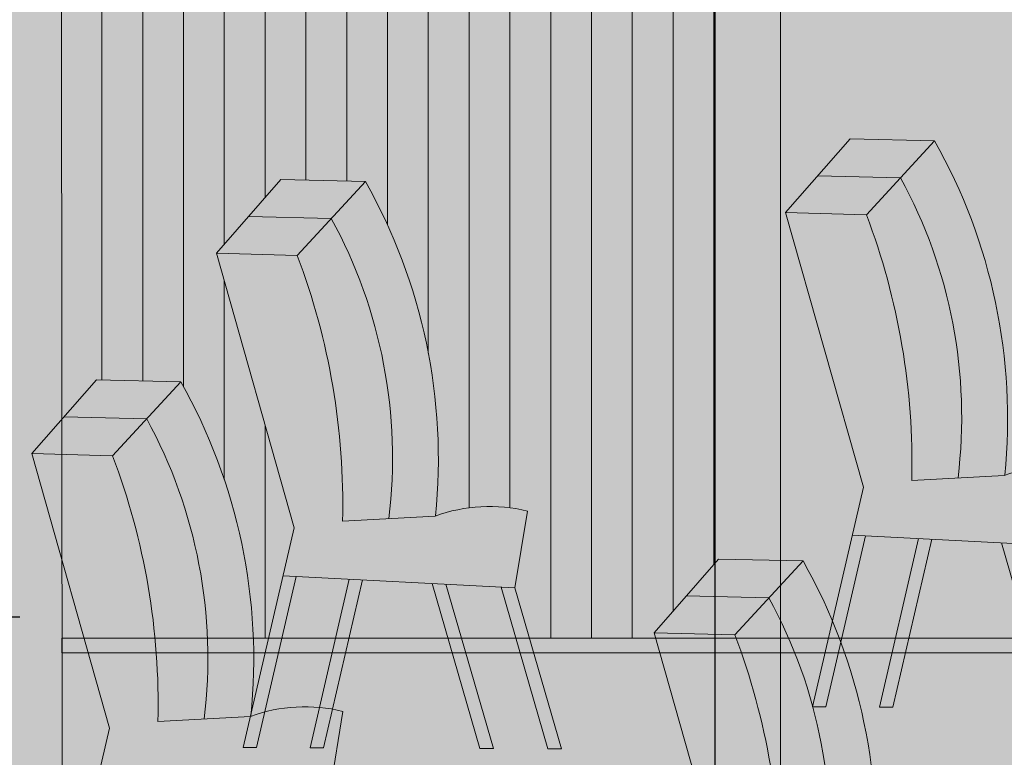
# Model space of a CAD drawing. Units: millimetres. Extents: x 11032 to 26788, y 3406 to 24505.
# Tile 8 of 78: x 15812 to 16566, y 7713 to 8278. Entities that reach past the tile are written whole.
import ezdxf

# ---------------------------------------------------------------- set-up
doc = ezdxf.new("R2010")
doc.units = ezdxf.units.MM
doc.header["$MEASUREMENT"] = 0
for name, color, linetype, lineweight in [('A-ANNO-DIMS', 2, 'Continuous', 18), ('A-FURN', 8, 'Continuous', 13), ('A-FURN-PATT', 8, 'Continuous', 13), ('A-GLAZ', 250, 'Continuous', 20), ('A-WALL-INTR', 8, 'Continuous', 18)]:
    doc.layers.add(name, color=color, linetype=linetype, lineweight=lineweight)
for name, color, linetype, lineweight, true_color in [('A-FNSH-INTR-PATT', 253, 'Continuous', 13, 0xc2b29b), ('A-GLAZ-FRAM-PATT', 250, 'Continuous', 13, 0x262627), ('A-WALL-INTR-PATT', 251, 'Continuous', 13, 0x6c6b6a)]:
    doc.layers.add(name, color=color, linetype=linetype, lineweight=lineweight, true_color=true_color)
doc.styles.get("Standard").update_dxf_attribs({"font": 'arial.ttf'})
doc.dimstyles.get("Standard").update_dxf_attribs({"dimtxt": 150, "dimasz": 100, "dimexe": 10, "dimexo": 5, "dimgap": 5, "dimtad": 0, "dimtih": 1, "dimtoh": 1, "dimdec": 0, "dimzin": 0, "dimdsep": 46, "dimtxsty": 'Standard', "dimcen": 0.09, "dimadec": 0, "dimazin": 0, "dimtfac": 1, "dimtdec": 0, "dimtofl": 0, "dimtmove": 0, "dimatfit": 3, "dimfxl": 1, "dimtolj": 1, "dimtzin": 0, "dimarcsym": 0})

# ---------------------------------------------------------------- blocks, each defined once
blk = doc.blocks.new('DINING-CHAIR-ELEV')
blk.add_line((228.68, 123.43), (51.04, 132.61))
for points in [[(0, 379.55), (49.45, 435.94), (114.12, 434.53)], [(61.18, 132.09), (30.79, 1.16), (20.53, 1.21), (59.55, 169.26), (0, 379.55), (61.9, 377.89)], [(111.9, 129.47), (82.06, 0.91), (71.8, 0.96), (101.76, 129.99)], [(165.28, 126.71), (201.76, 0.31), (212.19, 0.26), (175.85, 126.16)]]:
    blk.add_lwpolyline(points)
for points in [[(218.11, 123.98), (253.88, 0.05), (264.3, 0), (228.68, 123.43), (238.32, 182.18, 0.148451), (167.47, 178.33), (96.61, 174.48, 0.097012), (61.9, 377.89), (114.12, 434.53, -0.154833), (167.82, 178.46)], [(132.04, 176.4, 0.156877), (88.01, 406.21), (24.72, 407.74)]]:
    blk.add_lwpolyline(points, format="xyb")
blk = doc.blocks.new('DINING-TABLE-ELEV')
blk.add_lwpolyline([(0, 0), (986.08, 0), (986.08, 11.1), (0, 11.1)], close=True)
blk = doc.blocks.new('*D16')
at = {"layer": 'A-ANNO-DIMS', "color": 0, "lineweight": -2, "transparency": 16777216}
for p, q in [((15741.74, 7821.05), (15812.13, 7821.05)), ((15802.13, 7721.05), (15802.13, 7685.69)), ((15802.13, 7485.11), (15802.13, 7520.47)), ((15741.74, 7385.11), (15812.13, 7385.11))]:
    blk.add_line(p, q, dxfattribs=at)
at = {"layer": 'A-ANNO-DIMS', "color": 0, "transparency": 16777216}
for points in [[(15785.47, 7721.05), (15818.8, 7721.05), (15802.13, 7821.05)], [(15785.47, 7485.11), (15818.8, 7485.11), (15802.13, 7385.11)]]:
    blk.add_solid(points, dxfattribs=at)
at = {"layer": 'Defpoints', "color": 0, "transparency": 16777216}
for p in [(15736.74, 7821.05), (15802.13, 7821.05), (15736.74, 7385.11)]:
    blk.add_point(p, dxfattribs=at)
at = {"layer": 'A-ANNO-DIMS', "color": 0, "transparency": 16777216, "insert": (15802.13, 7603.08), "char_height": 150, "attachment_point": 5}
blk.add_mtext('\\A1;CHAIR 436 TYP.', dxfattribs=at)
blk = doc.blocks.new('*D36')
at = {"layer": 'A-ANNO-DIMS', "color": 0, "lineweight": -2, "transparency": 16777216}
for p, q in [((12301.26, 17115.89), (12301.26, 24416.86)), ((25397.4, 4466.4), (25397.4, 24416.86)), ((12401.26, 24406.86), (18569.2, 24406.86)), ((25297.4, 24406.86), (19129.47, 24406.86))]:
    blk.add_line(p, q, dxfattribs=at)
at = {"layer": 'A-ANNO-DIMS', "color": 0, "transparency": 16777216}
for points in [[(12401.26, 24423.52), (12401.26, 24390.19), (12301.26, 24406.86)], [(25297.4, 24423.52), (25297.4, 24390.19), (25397.4, 24406.86)]]:
    blk.add_solid(points, dxfattribs=at)
at = {"layer": 'Defpoints', "color": 0, "transparency": 16777216}
for p in [(25397.4, 24406.86), (12301.26, 17110.89), (25397.4, 4461.4)]:
    blk.add_point(p, dxfattribs=at)
at = {"layer": 'A-ANNO-DIMS', "color": 0, "transparency": 16777216, "insert": (18849.33, 24406.86), "char_height": 150, "attachment_point": 5}
blk.add_mtext('\\A1;13096', dxfattribs=at)
blk = doc.blocks.new('*D37')
at = {"layer": 'A-ANNO-DIMS', "color": 0, "lineweight": -2, "transparency": 16777216}
for p, q in [((18087.74, 23450.36), (11334.76, 23450.36)), ((11344.76, 23350.36), (11344.76, 14037.46)), ((11344.76, 4561.4), (11344.76, 13874.29)), ((12927.66, 4461.4), (11334.76, 4461.4))]:
    blk.add_line(p, q, dxfattribs=at)
at = {"layer": 'A-ANNO-DIMS', "color": 0, "transparency": 16777216}
for points in [[(11328.1, 23350.36), (11361.43, 23350.36), (11344.76, 23450.36)], [(11328.1, 4561.4), (11361.43, 4561.4), (11344.76, 4461.4)]]:
    blk.add_solid(points, dxfattribs=at)
at = {"layer": 'Defpoints', "color": 0, "transparency": 16777216}
for p in [(11344.76, 23450.36), (18092.74, 23450.36), (12932.66, 4461.4)]:
    blk.add_point(p, dxfattribs=at)
at = {"layer": 'A-ANNO-DIMS', "color": 0, "transparency": 16777216, "insert": (11344.76, 13955.88), "char_height": 150, "attachment_point": 5}
blk.add_mtext('\\A1;18989', dxfattribs=at)
blk = doc.blocks.new('*D49')
at = {"layer": 'A-ANNO-DIMS', "color": 0, "lineweight": -2, "transparency": 16777216}
for p, q in [((17953.45, 10206.41), (17953.45, 3494.9)), ((14996.4, 6406.4), (14996.4, 3494.9)), ((15096.4, 3504.9), (16244.67, 3504.9)), ((17853.45, 3504.9), (16705.18, 3504.9))]:
    blk.add_line(p, q, dxfattribs=at)
at = {"layer": 'A-ANNO-DIMS', "color": 0, "transparency": 16777216}
for points in [[(15096.4, 3521.57), (15096.4, 3488.23), (14996.4, 3504.9)], [(17853.45, 3521.57), (17853.45, 3488.23), (17953.45, 3504.9)]]:
    blk.add_solid(points, dxfattribs=at)
at = {"layer": 'Defpoints', "color": 0, "transparency": 16777216}
for p in [(17953.45, 10211.41), (14996.4, 6411.4), (17953.45, 3504.9)]:
    blk.add_point(p, dxfattribs=at)
at = {"layer": 'A-ANNO-DIMS', "color": 0, "transparency": 16777216, "insert": (16474.93, 3504.9), "char_height": 150, "attachment_point": 5}
blk.add_mtext('\\A1;2957', dxfattribs=at)
blk = doc.blocks.new('*D57')
at = {"layer": 'A-ANNO-DIMS', "color": 0, "lineweight": -2, "transparency": 16777216}
for p, q in [((14994.7, 7266.4), (14994.7, 24416.86)), ((20894.7, 7266.4), (20894.7, 24416.86)), ((15094.7, 24406.86), (17715.98, 24406.86)), ((20794.7, 24406.86), (18173.42, 24406.86))]:
    blk.add_line(p, q, dxfattribs=at)
at = {"layer": 'A-ANNO-DIMS', "color": 0, "transparency": 16777216}
for points in [[(15094.7, 24423.52), (15094.7, 24390.19), (14994.7, 24406.86)], [(20794.7, 24423.52), (20794.7, 24390.19), (20894.7, 24406.86)]]:
    blk.add_solid(points, dxfattribs=at)
at = {"layer": 'Defpoints', "color": 0, "transparency": 16777216}
for p in [(20894.7, 24406.86), (14994.7, 7261.4), (20894.7, 7261.4)]:
    blk.add_point(p, dxfattribs=at)
at = {"layer": 'A-ANNO-DIMS', "color": 0, "transparency": 16777216, "insert": (17944.7, 24406.86), "char_height": 150, "attachment_point": 5}
blk.add_mtext('\\A1;5900', dxfattribs=at)
blk = doc.blocks.new('*D60')
at = {"layer": 'A-ANNO-DIMS', "color": 0, "lineweight": -2, "transparency": 16777216}
for p, q in [((14994.7, 7266.4), (14994.7, 24416.86)), ((16344.7, 7266.4), (16344.7, 24416.86)), ((15094.7, 24406.86), (15448.04, 24406.86)), ((16244.7, 24406.86), (15891.36, 24406.86))]:
    blk.add_line(p, q, dxfattribs=at)
at = {"layer": 'A-ANNO-DIMS', "color": 0, "transparency": 16777216}
for points in [[(15094.7, 24423.52), (15094.7, 24390.19), (14994.7, 24406.86)], [(16244.7, 24423.52), (16244.7, 24390.19), (16344.7, 24406.86)]]:
    blk.add_solid(points, dxfattribs=at)
at = {"layer": 'Defpoints', "color": 0, "transparency": 16777216}
for p in [(16344.7, 24406.86), (14994.7, 7261.4), (16344.7, 7261.4)]:
    blk.add_point(p, dxfattribs=at)
at = {"layer": 'A-ANNO-DIMS', "color": 0, "transparency": 16777216, "insert": (15669.7, 24406.86), "char_height": 150, "attachment_point": 5}
blk.add_mtext('\\A1;1350', dxfattribs=at)
blk = doc.blocks.new('*D69')
at = {"layer": 'A-ANNO-DIMS', "color": 0, "lineweight": -2, "transparency": 16777216}
for p, q in [((13956.97, 9937.95), (14056.97, 9937.95)), ((14056.97, 9937.95), (15432.5, 8990.95)), ((17944.61, 7261.4), (17944.79, 7261.4)), ((17944.7, 7261.31), (17944.7, 7261.49))]:
    blk.add_line(p, q, dxfattribs=at)
at = {"layer": 'A-ANNO-DIMS', "color": 0, "transparency": 16777216}
blk.add_solid([(15441.95, 9004.68), (15423.05, 8977.22), (15514.87, 8934.24)], dxfattribs=at)
at = {"layer": 'Defpoints', "color": 0, "transparency": 16777216}
for p in [(15514.87, 8934.24), (17944.7, 7261.4)]:
    blk.add_point(p, dxfattribs=at)
at = {"layer": 'A-ANNO-DIMS', "color": 0, "transparency": 16777216, "insert": (13494.04, 9937.95), "char_height": 150, "attachment_point": 5}
blk.add_mtext('\\A1;2X R2950', dxfattribs=at)

msp = doc.modelspace()

# ---------------------------------------------------------------- hatches: boundary and pattern name
at = {"layer": 'A-FNSH-INTR-PATT'}
h = msp.add_hatch(dxfattribs=at)
h.set_pattern_fill('ANSI31', color=256, scale=250, angle=45, style=0)
h.paths.add_polyline_path([(16344.704, 9680.076, 0.0565356), (15843.607, 9260.247), (15844.323, 7974.176), (15846.037, 7974.134), (15870.762, 8002.329), (15935.434, 8000.923, -0.1195917), (15991.005, 7804.617), (16002.667, 7804.617), (16022.264, 7889.032), (15962.718, 8099.323), (16012.167, 8155.712), (16076.839, 8154.307, -0.1548334), (16130.535, 7898.229, -0.1476694), (16201.035, 7901.954), (16191.395, 7843.208), (16202.533, 7804.617), (16299.12, 7804.617), (16297.929, 7808.825), (16344.704, 7862.164)])
at = {"layer": 'A-FURN-PATT'}
h = msp.add_hatch(color=256, dxfattribs=at)
h.set_gradient(color1=(82, 15, 16), color2=(153, 0, 38), name='CURVED')
h.paths.add_polyline_path([(16952.125, 8119), (16926.017, 8147.32, 0.1568775), (16881.989, 7917.509), (16917.415, 7915.583, -0.0970121)], flags=0)
h.paths.add_polyline_path([(16899.908, 8175.64), (16964.58, 8177.046), (17014.03, 8120.657), (16954.484, 7910.365), (16972.017, 7834.84), (16977.75, 7834.965), (17027.199, 7778.576), (16967.653, 7568.284), (17006.665, 7400.238), (16996.411, 7400.187), (16966.016, 7531.114), (16925.439, 7529.018), (16955.395, 7399.983), (16945.141, 7399.932), (16915.295, 7528.494), (16861.916, 7525.736), (16825.435, 7399.337), (16815.012, 7399.285), (16851.35, 7525.19), (16809.087, 7523.007), (16773.319, 7399.078), (16762.896, 7399.026), (16798.521, 7522.461), (16788.882, 7581.207, -0.1476694), (16859.382, 7577.482, -0.1528132), (16911.41, 7830.579), (16902.125, 7870.575), (16848.746, 7867.817), (16830.506, 7804.617), (16830.506, 7793.515), (16827.302, 7793.515), (16812.265, 7741.418), (16801.842, 7741.366), (16816.893, 7793.515), (16775.261, 7793.515), (16760.15, 7741.159), (16749.727, 7741.107), (16764.853, 7793.515), (16650.704, 7793.515), (16662.994, 7750.932), (16652.571, 7750.983), (16640.296, 7793.515), (16598.663, 7793.515), (16610.879, 7751.191), (16600.455, 7751.242), (16588.255, 7793.515), (16490.425, 7793.515), (16480.749, 7751.837), (16470.495, 7751.888), (16480.159, 7793.515), (16443.833, 7793.515, -0.1094051), (16465.746, 7607.731, -0.1476694), (16536.246, 7611.456), (16526.606, 7552.71), (16562.232, 7429.275), (16551.809, 7429.327), (16516.041, 7553.255), (16473.778, 7555.439), (16510.116, 7429.534), (16499.693, 7429.586), (16463.212, 7555.985), (16409.833, 7558.743), (16379.987, 7430.181), (16369.733, 7430.232), (16394.704, 7537.793), (16394.704, 7559.524), (16359.112, 7561.363), (16328.717, 7430.435), (16318.463, 7430.486), (16344.704, 7543.521), (16344.704, 7643.635), (16302.264, 7793.515), (16205.738, 7793.515), (16227.021, 7719.773), (16216.598, 7719.825), (16195.329, 7793.515), (16153.697, 7793.515), (16174.905, 7720.032), (16164.482, 7720.084), (16143.289, 7793.515), (15844.423, 7793.515), (15844.423, 7804.617), (16140.084, 7804.617), (16128.001, 7846.483), (16191.395, 7843.208), (16201.035, 7901.954, 0.1484508), (16130.184, 7898.102), (16059.333, 7894.25, 0.0970121), (16024.622, 8097.666), (16076.839, 8154.307, -0.1548334), (16130.535, 7898.229, -0.1476694), (16201.035, 7901.954), (16191.395, 7843.208), (16202.533, 7804.617), (16299.12, 7804.617), (16297.929, 7808.825), (16347.378, 7865.214), (16412.05, 7863.808, -0.0295496), (16434.494, 7817.915), (16458.237, 7920.19), (16398.691, 8130.481), (16448.141, 8186.871), (16512.813, 8185.465, -0.1548334), (16566.508, 7929.387, -0.1476694), (16637.008, 7933.112), (16627.369, 7874.366), (16647.499, 7804.617), (16742.939, 7804.617), (16741.107, 8264.696), (17994.704, 8264.696), (17994.704, 7796.661), (18112.02, 7796.661), (18134.447, 7874.366), (18124.807, 7933.112, -0.1476694), (18195.307, 7929.387, -0.1548334), (18249.003, 8185.465), (18313.675, 8186.871), (18363.124, 8130.481), (18303.578, 7920.19), (18311.087, 7887.847, -0.0273017), (18332.016, 7930.161), (18396.688, 7931.567), (18446.137, 7875.177), (18423.905, 7796.661), (18470.25, 7796.661), (18470.25, 7785.559), (18420.761, 7785.559), (18386.591, 7664.886), (18425.604, 7496.839), (18415.35, 7496.788), (18384.955, 7627.716), (18344.377, 7625.62), (18374.333, 7496.584), (18364.079, 7496.533), (18334.233, 7625.095), (18280.854, 7622.338), (18244.373, 7495.938), (18233.95, 7495.887), (18270.288, 7621.792), (18228.026, 7619.608), (18192.257, 7495.679), (18181.834, 7495.628), (18217.46, 7619.062), (18207.82, 7677.808, -0.1476694), (18278.32, 7674.083, -0.0514181), (18278.516, 7762.821), (18273.237, 7785.559), (18171.265, 7785.559), (18161.36, 7751.242), (18150.937, 7751.191), (18160.856, 7785.559), (18119.224, 7785.559), (18109.244, 7750.983), (18098.821, 7750.932), (18108.815, 7785.559), (17852.794, 7785.559), (17866.18, 7739.181), (17855.756, 7739.233), (17842.386, 7785.559), (17800.753, 7785.559), (17814.064, 7739.44), (17803.641, 7739.492), (17790.345, 7785.559), (17694.491, 7785.559), (17685.986, 7748.922, -0.0882745), (17728.687, 7746.171), (17719.047, 7687.425), (17754.673, 7563.99), (17744.25, 7564.042), (17708.482, 7687.971), (17666.219, 7690.154), (17702.557, 7564.249), (17692.134, 7564.301), (17655.653, 7690.7), (17602.274, 7693.458), (17572.428, 7564.896), (17562.174, 7564.947), (17592.13, 7693.982), (17551.553, 7696.078), (17521.158, 7565.151), (17510.903, 7565.202), (17549.916, 7733.248), (17535.103, 7785.559), (17484.167, 7785.559), (17484.167, 7796.661), (17531.96, 7796.661), (17490.37, 7943.54), (17539.819, 7999.929), (17604.491, 7998.523, -0.0802486), (17652.289, 7869.096), (17661.422, 7908.439), (17601.876, 8118.731), (17651.326, 8175.12), (17715.998, 8173.714, -0.1548334), (17769.694, 7917.637, -0.1476694), (17840.194, 7921.361), (17830.554, 7862.615), (17849.59, 7796.661), (17894.704, 7796.661), (17894.704, 8239.696), (16741.207, 8239.696), (16742.939, 7804.617), (16768.057, 7804.617), (16785.352, 7864.542), (16775.713, 7923.288, -0.1476694), (16846.212, 7919.563, -0.1548334)], flags=17)
h.paths.add_polyline_path([(16899.908, 8175.64), (16964.58, 8177.046), (17014.03, 8120.657), (16954.484, 7910.365), (16993.496, 7742.318), (16983.242, 7742.267), (16952.847, 7873.195), (16912.27, 7871.099), (16942.225, 7742.064), (16931.971, 7742.013), (16902.125, 7870.575), (16848.746, 7867.817), (16812.265, 7741.418), (16801.842, 7741.366), (16838.181, 7867.271), (16795.918, 7865.087), (16760.15, 7741.159), (16749.727, 7741.107), (16785.352, 7864.542), (16775.713, 7923.288, -0.1476694), (16846.212, 7919.563, -0.1548334)], flags=0)
h.paths.add_polyline_path([(16899.908, 8175.64), (16964.58, 8177.046), (17014.03, 8120.657), (16954.484, 7910.365), (16972.017, 7834.84), (16977.75, 7834.965), (17027.199, 7778.576), (16967.653, 7568.284), (17006.665, 7400.238), (16996.411, 7400.187), (16966.016, 7531.114), (16925.439, 7529.018), (16955.395, 7399.983), (16945.141, 7399.932), (16915.295, 7528.494), (16861.916, 7525.736), (16825.435, 7399.337), (16815.012, 7399.285), (16851.35, 7525.19), (16809.087, 7523.007), (16773.319, 7399.078), (16762.896, 7399.026), (16798.521, 7522.461), (16788.882, 7581.207, -0.1476694), (16859.382, 7577.482, -0.1528132), (16911.41, 7830.579), (16902.125, 7870.575), (16848.746, 7867.817), (16830.506, 7804.617), (16830.506, 7793.515), (16827.302, 7793.515), (16812.265, 7741.418), (16801.842, 7741.366), (16816.893, 7793.515), (16775.261, 7793.515), (16760.15, 7741.159), (16749.727, 7741.107), (16764.853, 7793.515), (16650.704, 7793.515), (16662.994, 7750.932), (16652.571, 7750.983), (16640.296, 7793.515), (16598.663, 7793.515), (16610.879, 7751.191), (16600.455, 7751.242), (16588.255, 7793.515), (16490.425, 7793.515), (16480.749, 7751.837), (16470.495, 7751.888), (16480.159, 7793.515), (16443.833, 7793.515, -0.1094051), (16465.746, 7607.731, -0.1476694), (16536.246, 7611.456), (16526.606, 7552.71), (16562.232, 7429.275), (16551.809, 7429.327), (16516.041, 7553.255), (16473.778, 7555.439), (16510.116, 7429.534), (16499.693, 7429.586), (16463.212, 7555.985), (16409.833, 7558.743), (16379.987, 7430.181), (16369.733, 7430.232), (16394.704, 7537.793), (16394.704, 7559.524), (16359.112, 7561.363), (16328.717, 7430.435), (16318.463, 7430.486), (16344.704, 7543.521), (16344.704, 7643.635), (16302.264, 7793.515), (16205.738, 7793.515), (16227.021, 7719.773), (16216.598, 7719.825), (16195.329, 7793.515), (16153.697, 7793.515), (16174.905, 7720.032), (16164.482, 7720.084), (16143.289, 7793.515), (15844.423, 7793.515), (15844.423, 7804.617), (16140.084, 7804.617), (16128.001, 7846.483), (16191.395, 7843.208), (16201.035, 7901.954, 0.1484508), (16130.184, 7898.102), (16059.333, 7894.25, 0.0970121), (16024.622, 8097.666), (16076.839, 8154.307, -0.1548334), (16130.535, 7898.229, -0.1476694), (16201.035, 7901.954), (16191.395, 7843.208), (16202.533, 7804.617), (16299.12, 7804.617), (16297.929, 7808.825), (16347.378, 7865.214), (16412.05, 7863.808, -0.0295496), (16434.494, 7817.915), (16458.237, 7920.19), (16398.691, 8130.481), (16448.141, 8186.871), (16512.813, 8185.465, -0.1548334), (16566.508, 7929.387, -0.1476694), (16637.008, 7933.112), (16627.369, 7874.366), (16647.499, 7804.617), (16742.939, 7804.617), (16741.207, 8239.696), (16741.107, 8264.696), (17994.704, 8264.696), (17994.704, 7796.661), (18112.02, 7796.661), (18134.447, 7874.366), (18124.807, 7933.112, -0.1476694), (18195.307, 7929.387, -0.1548334), (18249.003, 8185.465), (18313.675, 8186.871), (18363.124, 8130.481), (18303.578, 7920.19), (18311.087, 7887.847, -0.0273017), (18332.016, 7930.161), (18396.688, 7931.567), (18446.137, 7875.177), (18423.905, 7796.661), (18470.25, 7796.661), (18470.25, 7785.559), (18420.761, 7785.559), (18386.591, 7664.886), (18425.604, 7496.839), (18415.35, 7496.788), (18384.955, 7627.716), (18344.377, 7625.62), (18374.333, 7496.584), (18364.079, 7496.533), (18334.233, 7625.095), (18280.854, 7622.338), (18244.373, 7495.938), (18233.95, 7495.887), (18270.288, 7621.792), (18228.026, 7619.608), (18192.257, 7495.679), (18181.834, 7495.628), (18217.46, 7619.062), (18207.82, 7677.808, -0.1476694), (18278.32, 7674.083, -0.0514181), (18278.516, 7762.821), (18273.237, 7785.559), (18171.265, 7785.559), (18161.36, 7751.242), (18150.937, 7751.191), (18160.856, 7785.559), (18119.224, 7785.559), (18109.244, 7750.983), (18098.821, 7750.932), (18108.815, 7785.559), (17852.794, 7785.559), (17866.18, 7739.181), (17855.756, 7739.233), (17842.386, 7785.559), (17800.753, 7785.559), (17814.064, 7739.44), (17803.641, 7739.492), (17790.345, 7785.559), (17694.491, 7785.559), (17685.986, 7748.922, -0.0882745), (17728.687, 7746.171), (17719.047, 7687.425), (17754.673, 7563.99), (17744.25, 7564.042), (17708.482, 7687.971), (17666.219, 7690.154), (17702.557, 7564.249), (17692.134, 7564.301), (17655.653, 7690.7), (17602.274, 7693.458), (17572.428, 7564.896), (17562.174, 7564.947), (17592.13, 7693.982), (17551.553, 7696.078), (17521.158, 7565.151), (17510.903, 7565.202), (17549.916, 7733.248), (17535.103, 7785.559), (17484.167, 7785.559), (17484.167, 7796.661), (17531.96, 7796.661), (17490.37, 7943.54), (17539.819, 7999.929), (17604.491, 7998.523, -0.0802486), (17652.289, 7869.096), (17661.422, 7908.439), (17601.876, 8118.731), (17651.326, 8175.12), (17715.998, 8173.714, -0.1548334), (17769.694, 7917.637, -0.1476694), (17840.194, 7921.361), (17830.554, 7862.615), (17849.59, 7796.661), (17894.704, 7796.661), (17894.704, 8239.696), (16741.207, 8239.696), (16742.939, 7804.617), (16768.057, 7804.617), (16785.352, 7864.542), (16775.713, 7923.288, -0.1476694), (16846.212, 7919.563, -0.1548334)], flags=17)
h = msp.add_hatch(color=256, dxfattribs=at)
h.set_gradient(color1=(153, 27, 30), color2=(153, 38, 0), name='SPHERICAL')
h.paths.add_polyline_path([(15534.344, 7763), (15472.44, 7764.657), (15531.986, 7554.365), (15523.479, 7517.719), (15640.736, 7511.661), (15653.713, 7567.556, 0.0295203), (15639.906, 7563.436), (15569.055, 7559.583, 0.0970121)], flags=16)
h.paths.add_polyline_path([(15560.453, 7791.32), (15534.344, 7763, -0.0970121), (15569.055, 7559.583), (15604.48, 7561.509, 0.1568775)], flags=16)
h.paths.add_polyline_path([(15586.562, 7819.64), (15560.453, 7791.32, -0.1568775), (15604.48, 7561.509), (15640.246, 7563.454, 0.154898)], flags=17)
h.paths.add_polyline_path([(15560.453, 7791.32), (15497.165, 7792.851), (15472.44, 7764.657), (15534.344, 7763)], flags=16)
h.paths.add_polyline_path([(15586.562, 7819.64), (15521.889, 7821.046), (15497.165, 7792.851), (15560.453, 7791.32)], flags=17)
h.paths.add_polyline_path([(15790.874, 7662.689, 0.021469), (15780.879, 7659.53), (15710.028, 7655.677, 0.0970121), (15675.317, 7859.094), (15665.772, 7859.35), (15665.799, 7675.745), (15672.959, 7650.459), (15665.807, 7619.654), (15665.808, 7613.744), (15790.755, 7607.288)], flags=17)
h.paths.add_polyline_path([(15665.772, 7859.35), (15613.413, 7860.751), (15665.799, 7675.745)], flags=16)
h.paths.add_polyline_path([(15701.426, 7887.414), (15665.767, 7888.277), (15665.772, 7859.35), (15675.317, 7859.094)], flags=16)
h.paths.add_polyline_path([(15727.534, 7915.735), (15665.763, 7917.077), (15665.767, 7888.277), (15701.426, 7887.414)], flags=17)
h.paths.add_polyline_path([(15665.763, 7917.077), (15662.862, 7917.14), (15638.137, 7888.946), (15665.767, 7888.277)], flags=17)
h.paths.add_polyline_path([(15665.767, 7888.277), (15638.137, 7888.946), (15613.413, 7860.751), (15665.772, 7859.35)], flags=16)
h.paths.add_polyline_path([(15701.426, 7887.414), (15675.317, 7859.094, -0.0970121), (15710.028, 7655.677), (15745.453, 7657.604, 0.1568775)], flags=16)
h.paths.add_polyline_path([(15844.495, 7664.925), (15844.384, 7864.461), (15821.312, 7945.94), (15870.762, 8002.329), (15935.434, 8000.923, -0.1195917), (15991.005, 7804.617), (16002.667, 7804.617), (16022.264, 7889.032), (15962.718, 8099.323), (16024.622, 8097.666), (16076.839, 8154.307, -0.1548334), (16130.535, 7898.229, -0.1476694), (16201.035, 7901.954), (16191.395, 7843.208), (16202.533, 7804.617), (16299.12, 7804.617), (16297.929, 7808.825), (16347.378, 7865.214), (16412.05, 7863.808, -0.0295496), (16434.494, 7817.915), (16458.237, 7920.19), (16398.691, 8130.481), (16460.595, 8128.825), (16512.813, 8185.465, -0.1548334), (16566.508, 7929.387, -0.1476694), (16637.008, 7933.112), (16627.369, 7874.366), (16647.499, 7804.617), (16830.506, 7804.617), (16830.506, 7793.515), (16650.704, 7793.515), (16662.994, 7750.932), (16652.571, 7750.983), (16640.296, 7793.515), (16490.425, 7793.515), (16480.749, 7751.837), (16470.495, 7751.888), (16480.159, 7793.515), (16443.833, 7793.515, -0.1094051), (16465.746, 7607.731, -0.1476694), (16536.246, 7611.456), (16526.606, 7552.71), (16562.232, 7429.275), (16551.809, 7429.327), (16516.041, 7553.255), (16473.778, 7555.439), (16510.116, 7429.534), (16499.693, 7429.586), (16463.212, 7555.985), (16409.833, 7558.743), (16379.987, 7430.181), (16369.733, 7430.232), (16394.704, 7537.793), (16394.704, 7559.524), (16359.112, 7561.363), (16328.717, 7430.435), (16318.463, 7430.486), (16344.704, 7543.521), (16344.704, 7643.635), (16302.264, 7793.515), (16205.738, 7793.515), (16227.021, 7719.773), (16216.598, 7719.825), (16195.329, 7793.515), (16153.697, 7793.515), (16174.905, 7720.032), (16164.482, 7720.084), (16143.289, 7793.515), (16061.685, 7793.515), (16051.641, 7750.248, -0.0167144), (16059.629, 7748.571), (16049.99, 7689.825), (16085.615, 7566.39), (16075.192, 7566.442), (16039.424, 7690.371), (15997.161, 7692.554), (16033.5, 7566.649), (16023.077, 7566.701), (15986.595, 7693.1), (15933.216, 7695.858), (15903.371, 7567.296), (15893.116, 7567.347), (15923.072, 7696.382), (15882.495, 7698.478), (15852.409, 7568.882), (15877.716, 7481.201), (15867.293, 7481.253), (15842.372, 7567.599), (15841.846, 7567.602), (15842.08, 7568.609), (15831.524, 7605.182), (15790.755, 7607.288), (15790.744, 7602.228), (15825.6, 7481.46), (15815.177, 7481.512), (15778.696, 7607.911), (15725.317, 7610.669), (15701.389, 7507.6), (15736.743, 7385.107), (15726.32, 7385.159), (15696.749, 7487.614), (15695.471, 7482.107), (15685.217, 7482.158), (15691.06, 7507.327), (15690.552, 7509.088), (15650.881, 7511.137), (15649.743, 7506.234), (15684.627, 7385.366), (15674.204, 7385.418), (15645.103, 7486.248), (15644.2, 7482.362), (15633.946, 7482.413), (15639.413, 7505.961), (15637.723, 7511.817), (15584.344, 7514.575), (15554.498, 7386.013), (15544.244, 7386.064), (15574.2, 7515.099), (15533.623, 7517.195), (15503.228, 7386.268), (15492.974, 7386.319), (15531.986, 7554.365), (15472.44, 7764.657), (15497.165, 7792.851), (15521.889, 7821.046), (15586.562, 7819.64, -0.1548334), (15640.257, 7563.563, -0.0287549), (15653.713, 7567.556), (15665.807, 7619.654), (15665.799, 7675.745), (15613.413, 7860.751), (15638.137, 7888.946), (15662.862, 7917.14), (15665.763, 7917.077), (15727.534, 7915.735, -0.1548334), (15781.23, 7659.657, -0.1322263)])
h = msp.add_hatch(color=256, dxfattribs=at)
h.set_gradient(color1=(153, 27, 30), color2=(153, 38, 0), name='SPHERICAL')
h.paths.add_polyline_path([(16050.731, 8125.986), (15987.442, 8127.518), (15962.718, 8099.323), (16024.622, 8097.666)])
h.paths.add_polyline_path([(16076.839, 8154.307), (16012.167, 8155.712), (15987.442, 8127.518), (16050.731, 8125.986)])
h.paths.add_polyline_path([(16486.704, 8157.145), (16423.416, 8158.676), (16398.691, 8130.481), (16460.595, 8128.825)])
h.paths.add_polyline_path([(16512.813, 8185.465), (16448.141, 8186.871), (16423.416, 8158.676), (16486.704, 8157.145)])
h = msp.add_hatch(color=256, dxfattribs=at)
h.set_gradient(color1=(153, 27, 30), color2=(153, 38, 0), name='SPHERICAL')
h.paths.add_polyline_path([(15710.028, 7655.677), (15745.453, 7657.604, 0.1568775), (15701.426, 7887.414), (15675.317, 7859.094, -0.0970121)], flags=16)
h.paths.add_polyline_path([(15790.755, 7607.288), (15790.874, 7662.689, 0.021469), (15780.879, 7659.53), (15710.028, 7655.677, 0.0970121), (15675.317, 7859.094), (15665.772, 7859.35), (15665.799, 7675.745), (15672.959, 7650.459), (15665.807, 7619.654), (15665.808, 7613.744)], flags=17)
h.paths.add_polyline_path([(15653.713, 7567.556), (15665.807, 7619.654), (15665.799, 7675.745), (15613.413, 7860.751), (15662.862, 7917.14), (15727.534, 7915.735, -0.1548334), (15781.23, 7659.657, -0.1322263), (15844.495, 7664.925), (15844.384, 7864.461), (15821.312, 7945.94), (15883.216, 7944.283), (15935.434, 8000.923, -0.1195917), (15991.005, 7804.617), (16002.667, 7804.617), (16022.264, 7889.032), (15962.718, 8099.323), (16024.622, 8097.666), (16076.839, 8154.307, -0.1548334), (16130.535, 7898.229, -0.1476694), (16201.035, 7901.954), (16191.395, 7843.208), (16202.533, 7804.617), (16830.506, 7804.617), (16830.506, 7793.515), (16205.738, 7793.515), (16227.021, 7719.773), (16216.598, 7719.825), (16195.329, 7793.515), (16153.697, 7793.515), (16174.905, 7720.032), (16164.482, 7720.084), (16143.289, 7793.515), (16061.685, 7793.515), (16051.641, 7750.248, -0.0167144), (16059.629, 7748.571), (16049.99, 7689.825), (16085.615, 7566.39), (16075.192, 7566.442), (16039.424, 7690.371), (15997.161, 7692.554), (16033.5, 7566.649), (16023.077, 7566.701), (15986.595, 7693.1), (15933.216, 7695.858), (15903.371, 7567.296), (15893.116, 7567.347), (15923.072, 7696.382), (15882.495, 7698.478), (15852.409, 7568.882), (15877.716, 7481.201), (15867.293, 7481.253), (15842.372, 7567.599), (15841.846, 7567.602), (15842.08, 7568.609), (15831.524, 7605.182), (15790.755, 7607.288), (15790.744, 7602.228), (15825.6, 7481.46), (15815.177, 7481.512), (15778.696, 7607.911), (15725.317, 7610.669), (15701.389, 7507.6), (15736.743, 7385.107), (15726.32, 7385.159), (15696.749, 7487.614), (15695.471, 7482.107), (15685.217, 7482.158), (15705.262, 7568.502, 0.0841685), (15664.448, 7569.579), (15644.2, 7482.362), (15633.946, 7482.413), (15653.713, 7567.556, 0.0295203), (15639.906, 7563.436), (15569.055, 7559.583, 0.0970121), (15534.344, 7763), (15472.44, 7764.657), (15521.889, 7821.046), (15586.562, 7819.64, -0.1548334), (15640.257, 7563.563, -0.0287549)])
at = {"layer": 'A-GLAZ-FRAM-PATT'}
h = msp.add_hatch(color=256, dxfattribs=at)
h.paths.add_polyline_path([(17944.704, 7311.399), (16344.704, 7311.399), (16344.704, 7261.399), (17944.704, 7261.399)], flags=17)
h.paths.add_polyline_path([(16344.704, 7311.399), (15045.135, 7311.399, -0.9829047), (20844.273, 7311.399), (19544.704, 7311.399), (19544.704, 7261.399), (20894.704, 7261.399, 0.5148441), (16985.951, 10051.255, 0.3202679), (14994.704, 7261.399), (16344.704, 7261.399)])
h.paths.add_polyline_path([(18744.704, 7311.399), (17944.704, 7311.399), (17944.704, 7261.399), (18744.704, 7261.399)], flags=17)
h.paths.add_polyline_path([(19544.704, 7311.399), (18744.704, 7311.399), (18744.704, 7261.399), (19544.704, 7261.399)], flags=17)
h.paths.add_polyline_path([(18694.704, 7361.399), (17994.704, 7361.399), (17994.704, 7311.399), (18694.704, 7311.399)], flags=17)
h.paths.add_polyline_path([(18744.704, 7361.399), (18694.704, 7361.399), (18694.704, 7311.399), (18744.704, 7311.399)], flags=17)
h.paths.add_polyline_path([(17194.704, 7361.399), (17144.704, 7361.399), (17144.704, 7311.399), (17194.704, 7311.399)], flags=17)
h.paths.add_polyline_path([(17431.432, 7361.399), (17194.704, 7361.399), (17194.704, 7311.399), (17431.699, 7311.399)], flags=17)
h.paths.add_polyline_path([(17894.704, 7361.399), (17431.432, 7361.399), (17431.699, 7311.399), (17894.704, 7311.399)], flags=17)
h.paths.add_polyline_path([(17944.704, 7361.399), (17894.704, 7361.399), (17894.704, 7311.399), (17944.704, 7311.399)], flags=17)
h.paths.add_polyline_path([(17994.704, 7361.399), (17944.704, 7361.399), (17944.704, 7311.399), (17994.704, 7311.399)], flags=17)
h = msp.add_hatch(color=256, dxfattribs=at)
h.paths.add_polyline_path([(16394.704, 9712.419, 0.0051337), (16344.704, 9680.076), (16344.704, 7862.164), (16347.378, 7865.214), (16394.704, 7864.185)])
h.paths.add_polyline_path([(17144.704, 10048.871, 0.0235225), (16886.403, 9961.399), (17094.704, 9961.399), (17094.704, 8264.696), (17144.704, 8264.696)])
h.paths.add_polyline_path([(18794.704, 9961.399), (19003.004, 9961.399, 0.0235225), (18744.704, 10048.871), (18744.704, 8264.696), (18794.704, 8264.696)])
h.paths.add_polyline_path([(19544.704, 9680.076, 0.0051337), (19494.704, 9712.419), (19494.704, 7793.43), (19544.704, 7793.43)])
h = msp.add_hatch(color=256, dxfattribs=at)
h.paths.add_polyline_path([(16734.609, 9896.863, 0.0333754), (16394.704, 9712.419), (16394.704, 7804.617), (16431.407, 7804.617), (16458.237, 7920.19), (16398.691, 8130.481), (16448.141, 8186.871), (16512.813, 8185.465, -0.1548334), (16566.508, 7929.387, -0.1476694), (16637.008, 7933.112), (16627.369, 7874.366), (16647.499, 7804.617), (16742.939, 7804.617)])
h.paths.add_polyline_path([(17094.704, 9961.399), (16886.403, 9961.399, 0.0142221), (16734.609, 9896.863), (16741.107, 8264.696), (17094.704, 8264.696)])
h.paths.add_polyline_path([(17417.202, 10027.292), (17194.704, 10011.399), (17194.704, 8264.696), (17426.61, 8264.696)])
h.paths.add_polyline_path([(17144.704, 8239.696), (17094.704, 8239.696), (17094.704, 7361.399), (16394.704, 7361.399), (16394.704, 7493.572), (16379.987, 7430.181), (16369.733, 7430.232), (16394.704, 7537.793), (16394.704, 7559.524), (16359.112, 7561.363), (16344.704, 7499.3), (16344.704, 7311.399), (17144.704, 7311.399)])
h.paths.add_polyline_path([(17194.704, 8239.696), (17144.704, 8239.696), (17144.704, 7361.399), (17194.704, 7361.399)])
at = {"layer": 'A-WALL-INTR-PATT'}
for points in [[(16344.704, 9680.076, 0.0565356), (15843.607, 9260.247), (15844.323, 7974.176), (15846.037, 7974.134), (15870.762, 8002.329), (15935.434, 8000.923, -0.1195917), (15991.005, 7804.617), (16002.667, 7804.617), (16022.264, 7889.032), (15962.718, 8099.323), (16012.167, 8155.712), (16076.839, 8154.307, -0.1548334), (16130.535, 7898.229, -0.1476694), (16201.035, 7901.954), (16191.395, 7843.208), (16202.533, 7804.617), (16299.12, 7804.617), (16297.929, 7808.825), (16344.704, 7862.164)], [(15843.607, 9260.247, 0.0062633), (15794.195, 9206.987), (15790.874, 7662.689, -0.1112179), (15844.495, 7664.925), (15844.384, 7864.461), (15821.312, 7945.94), (15844.324, 7972.181)]]:
    msp.add_hatch(color=256, dxfattribs=at).paths.add_polyline_path(points)
h = msp.add_hatch(color=256, dxfattribs=at)
h.paths.add_polyline_path([(15302.659, 8457.059, 0.0281002), (15185.248, 8153.253), (15233.282, 7717.599), (15314.374, 7311.399), (15467.334, 7311.399), (15381.661, 7740.545)])
h.paths.add_polyline_path([(16344.704, 7543.521), (16344.704, 7643.635), (16302.264, 7793.515), (16205.738, 7793.515), (16227.021, 7719.773), (16216.598, 7719.825), (16195.329, 7793.515), (16153.697, 7793.515), (16174.905, 7720.032), (16164.482, 7720.084), (16143.289, 7793.515), (16061.685, 7793.515), (16051.641, 7750.248, -0.0167144), (16059.629, 7748.571), (16049.99, 7689.825), (16085.615, 7566.39), (16075.192, 7566.442), (16039.424, 7690.371), (15997.161, 7692.554), (16033.5, 7566.649), (16023.077, 7566.701), (15986.595, 7693.1), (15933.216, 7695.858), (15903.371, 7567.296), (15893.116, 7567.347), (15923.072, 7696.382), (15882.495, 7698.478), (15852.409, 7568.882), (15877.716, 7481.201), (15867.293, 7481.253), (15844.553, 7560.041), (15844.691, 7311.399), (16344.704, 7311.399), (16344.704, 7499.3), (16328.717, 7430.435), (16318.463, 7430.486)])
h.paths.add_polyline_path([(16742.983, 7793.515), (16650.704, 7793.515), (16662.994, 7750.932), (16652.571, 7750.983), (16640.296, 7793.515), (16598.663, 7793.515), (16610.879, 7751.191), (16600.455, 7751.242), (16588.255, 7793.515), (16490.425, 7793.515), (16480.749, 7751.837), (16470.495, 7751.888), (16480.159, 7793.515), (16443.833, 7793.515, -0.1094051), (16465.746, 7607.731, -0.1476694), (16536.246, 7611.456), (16526.606, 7552.71), (16562.232, 7429.275), (16551.809, 7429.327), (16516.041, 7553.255), (16473.778, 7555.439), (16510.116, 7429.534), (16499.693, 7429.586), (16463.212, 7555.985), (16409.833, 7558.743), (16394.704, 7493.572), (16394.704, 7361.399), (16744.704, 7361.399)])
h.paths.add_polyline_path([(17094.704, 8239.696), (16741.207, 8239.696), (16742.939, 7804.617), (16768.057, 7804.617), (16785.352, 7864.542), (16775.713, 7923.288, -0.1476694), (16846.212, 7919.563, -0.1548334), (16899.908, 8175.64), (16964.58, 8177.046), (17014.03, 8120.657), (16954.484, 7910.365), (16972.017, 7834.84), (16977.75, 7834.965), (17027.199, 7778.576), (16967.653, 7568.284), (17006.665, 7400.238), (16996.411, 7400.187), (16966.016, 7531.114), (16925.439, 7529.018), (16955.395, 7399.983), (16945.141, 7399.932), (16915.295, 7528.494), (16861.916, 7525.736), (16825.435, 7399.337), (16815.012, 7399.285), (16851.35, 7525.19), (16809.087, 7523.007), (16773.319, 7399.078), (16762.896, 7399.026), (16798.521, 7522.461), (16788.882, 7581.207, -0.1476694), (16859.382, 7577.482, -0.1528132), (16911.41, 7830.579), (16902.125, 7870.575), (16848.746, 7867.817), (16830.506, 7804.617), (16830.506, 7793.515), (16827.302, 7793.515), (16812.265, 7741.418), (16801.842, 7741.366), (16816.893, 7793.515), (16775.261, 7793.515), (16760.15, 7741.159), (16749.727, 7741.107), (16764.853, 7793.515), (16742.983, 7793.515), (16744.704, 7361.399), (17094.704, 7361.399)])
h.paths.add_polyline_path([(18950.929, 7931.023), (19015.601, 7932.429), (19065.05, 7876.04), (19005.504, 7665.748), (19014.012, 7629.102, -0.129191), (19069.892, 7841.762), (19134.564, 7843.167), (19168.958, 7803.946), (19202.145, 7841.791), (19246.92, 7840.817), (19212.932, 7960.847), (19262.382, 8017.236), (19327.054, 8015.831, -0.134919), (19382.824, 7793.43), (19562.845, 7793.43, -0.1257757), (19618.686, 8000.275), (19683.358, 8001.68), (19732.808, 7945.291), (19689.807, 7793.43), (19753.644, 7793.43, -0.0966843), (19805.964, 7950.707), (19870.637, 7952.112), (19920.086, 7895.723), (19891.121, 7793.43), (20039.255, 7793.43, -0.0897865), (20089.9, 7938.993), (20154.572, 7940.399), (20204.021, 7884.01), (20144.475, 7673.718), (20152.983, 7637.072, -0.1476694), (20223.483, 7633.347, -0.1548334), (20277.178, 7889.425), (20341.85, 7890.831), (20391.3, 7834.441), (20331.754, 7624.15), (20370.766, 7456.103), (20360.512, 7456.052), (20330.117, 7586.98), (20289.54, 7584.884), (20319.496, 7455.848), (20309.241, 7455.797), (20279.396, 7584.359), (20226.017, 7581.602), (20189.536, 7455.202), (20179.112, 7455.151), (20215.451, 7581.056), (20173.188, 7578.872), (20169.478, 7566.018), (20183.488, 7505.671), (20173.234, 7505.62), (20163.789, 7546.305), (20137.42, 7454.943), (20126.997, 7454.892), (20159.149, 7566.291), (20142.839, 7636.548), (20102.261, 7634.452), (20132.217, 7505.417), (20121.963, 7505.366), (20092.117, 7633.928), (20038.738, 7631.17), (20002.257, 7504.771), (19991.834, 7504.719), (20028.172, 7630.624), (19985.91, 7628.44), (19950.141, 7504.512), (19939.718, 7504.46), (19975.344, 7627.895), (19965.704, 7686.641, -0.1476694), (20036.204, 7682.916, -0.0576487), (20037.659, 7782.328), (19887.977, 7782.328), (19860.54, 7685.431), (19899.552, 7517.385), (19889.298, 7517.334), (19858.903, 7648.261), (19818.326, 7646.165), (19848.282, 7517.13), (19838.028, 7517.079), (19808.182, 7645.641), (19754.803, 7642.883), (19718.322, 7516.484), (19707.899, 7516.432), (19744.237, 7642.337), (19701.974, 7640.154), (19698.264, 7627.3), (19712.274, 7566.953), (19702.02, 7566.902), (19692.575, 7607.587), (19666.206, 7516.225), (19655.783, 7516.173), (19687.935, 7627.573), (19671.625, 7697.83), (19631.048, 7695.733), (19661.003, 7566.698), (19650.749, 7566.647), (19620.903, 7695.209), (19567.524, 7692.451), (19531.043, 7566.052), (19520.62, 7566), (19556.959, 7691.905), (19514.696, 7689.722), (19478.928, 7565.793), (19468.505, 7565.741), (19473, 7581.318), (19466.812, 7581.349), (19431.044, 7705.278), (19388.781, 7707.461), (19425.12, 7581.556), (19414.696, 7581.608), (19378.215, 7708.007), (19324.836, 7710.765), (19318.877, 7685.094, -0.0584523), (19320.513, 7584.307, -0.1476694), (19391.013, 7588.032), (19381.373, 7529.286), (19416.999, 7405.852), (19406.576, 7405.903), (19370.808, 7529.832), (19328.545, 7532.016), (19364.883, 7406.111), (19354.46, 7406.162), (19317.979, 7532.562), (19264.6, 7535.319), (19234.754, 7406.757), (19224.5, 7406.808), (19254.456, 7535.844), (19213.879, 7537.94), (19183.484, 7407.012), (19173.23, 7407.063), (19212.242, 7575.11), (19168.16, 7730.789), (19124.467, 7576.487), (19163.48, 7408.44), (19153.225, 7408.389), (19122.83, 7539.317), (19082.253, 7537.22), (19112.209, 7408.185), (19101.955, 7408.134), (19072.109, 7536.696), (19035.898, 7534.825), (19044.517, 7497.701), (19034.262, 7497.65), (19025.754, 7534.301), (19018.73, 7533.938), (18982.249, 7407.539), (18971.826, 7407.487), (19008.164, 7533.392), (18985.177, 7532.205), (18993.246, 7497.447), (18982.992, 7497.396), (18975.033, 7531.681), (18965.902, 7531.209), (18930.133, 7407.28), (18919.71, 7407.228), (18955.336, 7530.663), (18945.696, 7589.409, -0.0318483), (18960.996, 7592.142), (18953.146, 7625.958), (18899.767, 7623.2), (18863.286, 7496.801), (18852.863, 7496.749), (18889.201, 7622.654), (18846.938, 7620.47), (18811.17, 7496.542), (18800.747, 7496.49), (18836.373, 7619.924), (18826.733, 7678.67, -0.1476694), (18897.233, 7674.946, -0.1548334)], flags=16)

# ---------------------------------------------------------------- linework, layer by layer
at = {"layer": 'A-GLAZ'}
for p, q in [((16394.704, 7361.399), (16394.704, 9712.419)), ((16344.704, 7261.399), (16344.704, 9680.076))]:
    msp.add_line(p, q, dxfattribs=at)
for radius, start, end in [(2900, 0.987907, 179.012093), (2950, 108.965621, 181.942602)]:
    msp.add_arc((17944.704, 7261.399), radius, start, end, dxfattribs=at)
at = {"layer": 'A-WALL-INTR'}
msp.add_line((15843.607, 9260.247), (15844.691, 7311.399), dxfattribs=at)

# ---------------------------------------------------------------- block references
at = {"layer": 'A-FURN'}
for name, p in [('DINING-CHAIR-ELEV', (16398.691, 7750.932)), ('DINING-CHAIR-ELEV', (15962.718, 7719.773)), ('DINING-CHAIR-ELEV', (15821.312, 7566.39)), ('DINING-CHAIR-ELEV', (15613.413, 7481.201)), ('DINING-CHAIR-ELEV', (16297.929, 7429.275)), ('DINING-TABLE-ELEV', (15844.423, 7793.515))]:
    msp.add_blockref(name, p, dxfattribs=at)

# ---------------------------------------------------------------- dimensions: what is measured, and where the dimension line sits
at = {"layer": 'A-ANNO-DIMS'}
for base, p1, p2, picture, middle in [((25397.404, 24406.858), (12301.265, 17110.885), (25397.404, 4461.399), '*D36', (18849.334, 24406.858)), ((20894.704, 24406.858), (14994.704, 7261.399), (20894.704, 7261.399), '*D57', (17944.704, 24406.858)), ((16344.704, 24406.858), (14994.704, 7261.399), (16344.704, 7261.399), '*D60', (15669.704, 24406.858)), ((17953.455, 3504.899), (14996.399, 6411.399), (17953.455, 10211.41), '*D49', (16474.927, 3504.899))]:
    dim = msp.add_linear_dim(base=base, p1=p1, p2=p2, dimstyle='Standard', override={"dimdec": 0, "dimlfac": 1, "dimrnd": 0, "dimzin": 0, "dimdsep": 46, "dimlunit": 2}, dxfattribs=at)
    dim.commit()
    dim.dimension.update_dxf_attribs({"geometry": picture, "text_midpoint": middle})
dim = msp.add_linear_dim(base=(11344.765, 23450.358), p1=(12932.665, 4461.399), p2=(18092.739, 23450.358), angle=90, dimstyle='Standard', override={"dimdec": 0, "dimlfac": 1, "dimrnd": 0, "dimzin": 0, "dimdsep": 46, "dimlunit": 2}, dxfattribs=at)
dim.commit()
dim.dimension.update_dxf_attribs({"geometry": '*D37', "text_midpoint": (11344.765, 13955.879)})
dim = msp.add_radius_dim(center=(17944.704, 7261.399), mpoint=(15514.87, 8934.244), text='2X <>', dimstyle='Standard', override={"dimdec": 0, "dimlfac": 1, "dimrnd": 0, "dimzin": 0, "dimdsep": 46, "dimlunit": 2}, dxfattribs=at)
dim.commit()
dim.dimension.update_dxf_attribs({"geometry": '*D69', "text_midpoint": (13494.04, 9937.951), "dimtype": 164})
dim = msp.add_linear_dim(base=(15802.134, 7821.046), p1=(15736.743, 7385.107), p2=(15736.743, 7821.046), angle=90, text='CHAIR <> TYP.', dimstyle='Standard', override={"dimdec": 0, "dimlfac": 1, "dimrnd": 0, "dimzin": 0, "dimdsep": 46, "dimlunit": 2}, dxfattribs=at)
dim.commit()
dim.dimension.update_dxf_attribs({"geometry": '*D16', "text_midpoint": (15802.134, 7603.076)})

doc.saveas('drawing.dxf')
